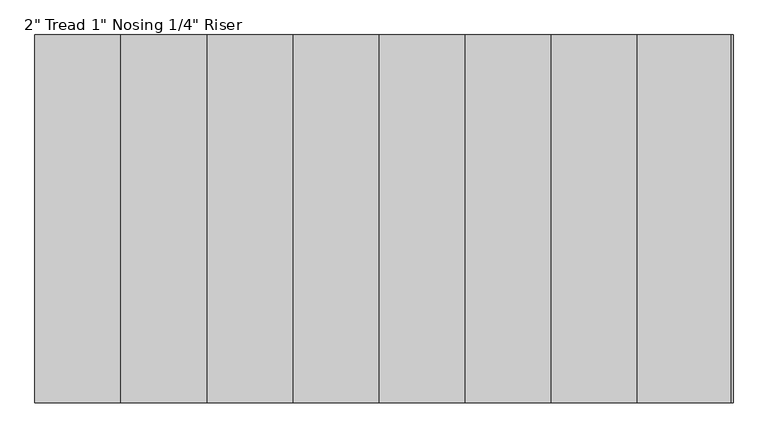
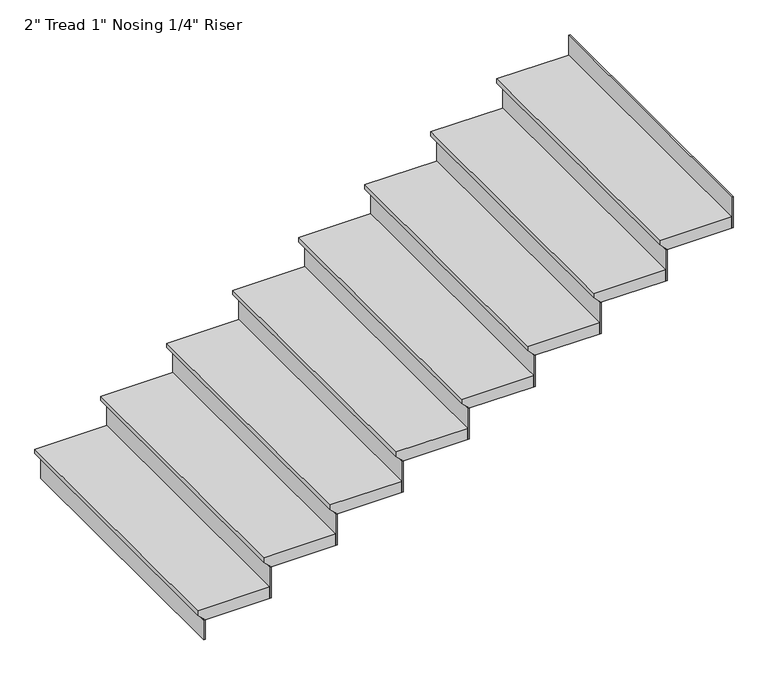
"""IFC4 building model written with IfcOpenShell, lengths in millimetres: stair flight geometry."""

from ifc_helpers import new_model, si_unit, origin, place, context, project, spatial, faceted_brep, source, transform, mapped, element, save


def stair_flight_e1fa31a4(model_context):
    return source(origin(), model_context, "Body", "Brep", [
        faceted_brep([(-12169.2183666, 2189.9503619, 3598.7934783), (-12169.2183666, 2189.9503619, 3617.8434783), (-12169.2183666, 3383.7503619, 3617.8434783), (-12169.2183666, 3383.7503619, 3598.7934783), (-12143.8183666, 2189.9503619, 3573.3934783), (-12143.8183666, 3383.7503619, 3573.3934783), (-11864.4183666, 2189.9503619, 3617.8434783), (-11864.4183666, 3383.7503619, 3617.8434783), (-12143.8183666, 3383.7503619, 3567.0434783), (-11864.4183666, 3383.7503619, 3567.0434783), (-11864.4183666, 2189.9503619, 3567.0434783), (-12143.8183666, 2189.9503619, 3567.0434783)], [[[0, 1, 2, 3]], [[4, 0, 3, 5]], [[2, 1, 6, 7]], [[8, 9, 10, 11]], [[2, 7, 9, 8, 5, 3]], [[8, 11, 4, 5]], [[6, 1, 0, 4, 11, 10]], [[7, 6, 10, 9]]]),
        faceted_brep([(-12143.8183666, 2189.9503619, 3567.0434783), (-12143.8183666, 2189.9503619, 3478.6956522), (-12137.4683666, 2189.9503619, 3478.6956522), (-12137.4683666, 2189.9503619, 3567.0434783), (-12143.8183666, 3383.7503619, 3567.0434783), (-12137.4683666, 3383.7503619, 3567.0434783), (-12137.4683666, 3383.7503619, 3478.6956522), (-12143.8183666, 3383.7503619, 3478.6956522)], [[[0, 1, 2, 3]], [[4, 5, 6, 7]], [[1, 0, 4, 7]], [[2, 1, 7, 6]], [[3, 2, 6, 5]], [[0, 3, 5, 4]]]),
        faceted_brep([(-11864.4183666, 2189.9503619, 3706.1913043), (-11864.4183666, 2189.9503619, 3567.0434783), (-11858.0683666, 2189.9503619, 3567.0434783), (-11858.0683666, 2189.9503619, 3706.1913043), (-11864.4183666, 3383.7503619, 3706.1913043), (-11858.0683666, 3383.7503619, 3706.1913043), (-11858.0683666, 3383.7503619, 3567.0434783), (-11864.4183666, 3383.7503619, 3567.0434783)], [[[0, 1, 2, 3]], [[4, 5, 6, 7]], [[1, 0, 4, 7]], [[2, 1, 7, 6]], [[3, 2, 6, 5]], [[0, 3, 5, 4]]]),
        faceted_brep([(-11889.8183666, 3383.7503619, 3756.9913043), (-11889.8183666, 2189.9503619, 3756.9913043), (-11585.0183666, 2189.9503619, 3756.9913043), (-11585.0183666, 3383.7503619, 3756.9913043), (-11864.4183666, 3383.7503619, 3706.1913043), (-11585.0183666, 3383.7503619, 3706.1913043), (-11585.0183666, 2189.9503619, 3706.1913043), (-11864.4183666, 2189.9503619, 3706.1913043), (-11864.4183666, 3383.7503619, 3712.5413043), (-11889.8183666, 3383.7503619, 3737.9413043), (-11864.4183666, 2189.9503619, 3712.5413043), (-11889.8183666, 2189.9503619, 3737.9413043)], [[[0, 1, 2, 3]], [[4, 5, 6, 7]], [[0, 3, 5, 4, 8, 9]], [[4, 7, 10, 8]], [[2, 1, 11, 10, 7, 6]], [[3, 2, 6, 5]], [[11, 1, 0, 9]], [[10, 11, 9, 8]]]),
        faceted_brep([(-11585.0183666, 2189.9503619, 3845.3391304), (-11585.0183666, 2189.9503619, 3706.1913043), (-11578.6683666, 2189.9503619, 3706.1913043), (-11578.6683666, 2189.9503619, 3845.3391304), (-11585.0183666, 3383.7503619, 3845.3391304), (-11578.6683666, 3383.7503619, 3845.3391304), (-11578.6683666, 3383.7503619, 3706.1913043), (-11585.0183666, 3383.7503619, 3706.1913043)], [[[0, 1, 2, 3]], [[4, 5, 6, 7]], [[1, 0, 4, 7]], [[2, 1, 7, 6]], [[3, 2, 6, 5]], [[0, 3, 5, 4]]]),
        faceted_brep([(-11610.4183666, 3383.7503619, 3896.1391304), (-11610.4183666, 2189.9503619, 3896.1391304), (-11305.6183666, 2189.9503619, 3896.1391304), (-11305.6183666, 3383.7503619, 3896.1391304), (-11585.0183666, 3383.7503619, 3845.3391304), (-11305.6183666, 3383.7503619, 3845.3391304), (-11305.6183666, 2189.9503619, 3845.3391304), (-11585.0183666, 2189.9503619, 3845.3391304), (-11585.0183666, 3383.7503619, 3851.6891304), (-11610.4183666, 3383.7503619, 3877.0891304), (-11585.0183666, 2189.9503619, 3851.6891304), (-11610.4183666, 2189.9503619, 3877.0891304)], [[[0, 1, 2, 3]], [[4, 5, 6, 7]], [[0, 3, 5, 4, 8, 9]], [[4, 7, 10, 8]], [[2, 1, 11, 10, 7, 6]], [[3, 2, 6, 5]], [[11, 1, 0, 9]], [[10, 11, 9, 8]]]),
        faceted_brep([(-11305.6183666, 2189.9503619, 3984.4869565), (-11305.6183666, 2189.9503619, 3845.3391304), (-11299.2683666, 2189.9503619, 3845.3391304), (-11299.2683666, 2189.9503619, 3984.4869565), (-11305.6183666, 3383.7503619, 3984.4869565), (-11299.2683666, 3383.7503619, 3984.4869565), (-11299.2683666, 3383.7503619, 3845.3391304), (-11305.6183666, 3383.7503619, 3845.3391304)], [[[0, 1, 2, 3]], [[4, 5, 6, 7]], [[1, 0, 4, 7]], [[2, 1, 7, 6]], [[3, 2, 6, 5]], [[0, 3, 5, 4]]]),
        faceted_brep([(-11331.0183666, 3383.7503619, 4035.2869565), (-11331.0183666, 2189.9503619, 4035.2869565), (-11026.2183666, 2189.9503619, 4035.2869565), (-11026.2183666, 3383.7503619, 4035.2869565), (-11305.6183666, 3383.7503619, 3984.4869565), (-11026.2183666, 3383.7503619, 3984.4869565), (-11026.2183666, 2189.9503619, 3984.4869565), (-11305.6183666, 2189.9503619, 3984.4869565), (-11305.6183666, 3383.7503619, 3990.8369565), (-11331.0183666, 3383.7503619, 4016.2369565), (-11305.6183666, 2189.9503619, 3990.8369565), (-11331.0183666, 2189.9503619, 4016.2369565)], [[[0, 1, 2, 3]], [[4, 5, 6, 7]], [[0, 3, 5, 4, 8, 9]], [[4, 7, 10, 8]], [[2, 1, 11, 10, 7, 6]], [[3, 2, 6, 5]], [[11, 1, 0, 9]], [[10, 11, 9, 8]]]),
        faceted_brep([(-11026.2183666, 2189.9503619, 4123.6347826), (-11026.2183666, 2189.9503619, 3984.4869565), (-11019.8683666, 2189.9503619, 3984.4869565), (-11019.8683666, 2189.9503619, 4123.6347826), (-11026.2183666, 3383.7503619, 4123.6347826), (-11019.8683666, 3383.7503619, 4123.6347826), (-11019.8683666, 3383.7503619, 3984.4869565), (-11026.2183666, 3383.7503619, 3984.4869565)], [[[0, 1, 2, 3]], [[4, 5, 6, 7]], [[1, 0, 4, 7]], [[2, 1, 7, 6]], [[3, 2, 6, 5]], [[0, 3, 5, 4]]]),
        faceted_brep([(-11051.6183666, 3383.7503619, 4174.4347826), (-11051.6183666, 2189.9503619, 4174.4347826), (-10746.8183666, 2189.9503619, 4174.4347826), (-10746.8183666, 3383.7503619, 4174.4347826), (-11026.2183666, 3383.7503619, 4123.6347826), (-10746.8183666, 3383.7503619, 4123.6347826), (-10746.8183666, 2189.9503619, 4123.6347826), (-11026.2183666, 2189.9503619, 4123.6347826), (-11026.2183666, 3383.7503619, 4129.9847826), (-11051.6183666, 3383.7503619, 4155.3847826), (-11026.2183666, 2189.9503619, 4129.9847826), (-11051.6183666, 2189.9503619, 4155.3847826)], [[[0, 1, 2, 3]], [[4, 5, 6, 7]], [[0, 3, 5, 4, 8, 9]], [[4, 7, 10, 8]], [[2, 1, 11, 10, 7, 6]], [[3, 2, 6, 5]], [[11, 1, 0, 9]], [[10, 11, 9, 8]]]),
        faceted_brep([(-10746.8183666, 2189.9503619, 4262.7826087), (-10746.8183666, 2189.9503619, 4123.6347826), (-10740.4683666, 2189.9503619, 4123.6347826), (-10740.4683666, 2189.9503619, 4262.7826087), (-10746.8183666, 3383.7503619, 4262.7826087), (-10740.4683666, 3383.7503619, 4262.7826087), (-10740.4683666, 3383.7503619, 4123.6347826), (-10746.8183666, 3383.7503619, 4123.6347826)], [[[0, 1, 2, 3]], [[4, 5, 6, 7]], [[1, 0, 4, 7]], [[2, 1, 7, 6]], [[3, 2, 6, 5]], [[0, 3, 5, 4]]]),
        faceted_brep([(-10772.2183666, 3383.7503619, 4313.5826087), (-10772.2183666, 2189.9503619, 4313.5826087), (-10467.4183666, 2189.9503619, 4313.5826087), (-10467.4183666, 3383.7503619, 4313.5826087), (-10746.8183666, 3383.7503619, 4262.7826087), (-10467.4183666, 3383.7503619, 4262.7826087), (-10467.4183666, 2189.9503619, 4262.7826087), (-10746.8183666, 2189.9503619, 4262.7826087), (-10746.8183666, 3383.7503619, 4269.1326087), (-10772.2183666, 3383.7503619, 4294.5326087), (-10746.8183666, 2189.9503619, 4269.1326087), (-10772.2183666, 2189.9503619, 4294.5326087)], [[[0, 1, 2, 3]], [[4, 5, 6, 7]], [[0, 3, 5, 4, 8, 9]], [[4, 7, 10, 8]], [[2, 1, 11, 10, 7, 6]], [[3, 2, 6, 5]], [[11, 1, 0, 9]], [[10, 11, 9, 8]]]),
        faceted_brep([(-10467.4183666, 2189.9503619, 4401.9304348), (-10467.4183666, 2189.9503619, 4262.7826087), (-10461.0683666, 2189.9503619, 4262.7826087), (-10461.0683666, 2189.9503619, 4401.9304348), (-10467.4183666, 3383.7503619, 4401.9304348), (-10461.0683666, 3383.7503619, 4401.9304348), (-10461.0683666, 3383.7503619, 4262.7826087), (-10467.4183666, 3383.7503619, 4262.7826087)], [[[0, 1, 2, 3]], [[4, 5, 6, 7]], [[1, 0, 4, 7]], [[2, 1, 7, 6]], [[3, 2, 6, 5]], [[0, 3, 5, 4]]]),
        faceted_brep([(-10492.8183666, 3383.7503619, 4452.7304348), (-10492.8183666, 2189.9503619, 4452.7304348), (-10188.0183666, 2189.9503619, 4452.7304348), (-10188.0183666, 3383.7503619, 4452.7304348), (-10467.4183666, 3383.7503619, 4401.9304348), (-10188.0183666, 3383.7503619, 4401.9304348), (-10188.0183666, 2189.9503619, 4401.9304348), (-10467.4183666, 2189.9503619, 4401.9304348), (-10467.4183666, 3383.7503619, 4408.2804348), (-10492.8183666, 3383.7503619, 4433.6804348), (-10467.4183666, 2189.9503619, 4408.2804348), (-10492.8183666, 2189.9503619, 4433.6804348)], [[[0, 1, 2, 3]], [[4, 5, 6, 7]], [[0, 3, 5, 4, 8, 9]], [[4, 7, 10, 8]], [[2, 1, 11, 10, 7, 6]], [[3, 2, 6, 5]], [[11, 1, 0, 9]], [[10, 11, 9, 8]]]),
        faceted_brep([(-10188.0183666, 2189.9503619, 4541.0782609), (-10188.0183666, 2189.9503619, 4401.9304348), (-10181.6683666, 2189.9503619, 4401.9304348), (-10181.6683666, 2189.9503619, 4541.0782609), (-10188.0183666, 3383.7503619, 4541.0782609), (-10181.6683666, 3383.7503619, 4541.0782609), (-10181.6683666, 3383.7503619, 4401.9304348), (-10188.0183666, 3383.7503619, 4401.9304348)], [[[0, 1, 2, 3]], [[4, 5, 6, 7]], [[1, 0, 4, 7]], [[2, 1, 7, 6]], [[3, 2, 6, 5]], [[0, 3, 5, 4]]]),
        faceted_brep([(-9908.6183666, 2189.9503619, 4680.226087), (-9908.6183666, 2189.9503619, 4541.0782609), (-9902.2683666, 2189.9503619, 4541.0782609), (-9902.2683666, 2189.9503619, 4680.226087), (-9908.6183666, 3383.7503619, 4680.226087), (-9902.2683666, 3383.7503619, 4680.226087), (-9902.2683666, 3383.7503619, 4541.0782609), (-9908.6183666, 3383.7503619, 4541.0782609)], [[[0, 1, 2, 3]], [[4, 5, 6, 7]], [[1, 0, 4, 7]], [[2, 1, 7, 6]], [[3, 2, 6, 5]], [[0, 3, 5, 4]]]),
        faceted_brep([(-9908.6183666, 3383.7503619, 4591.8782609), (-9934.0183666, 3383.7503619, 4591.8782609), (-10213.4183666, 3383.7503619, 4591.8782609), (-10213.4183666, 2189.9503619, 4591.8782609), (-9908.6183666, 2189.9503619, 4591.8782609), (-9934.0183666, 3383.7503619, 4541.0782609), (-9908.6183666, 3383.7503619, 4541.0782609), (-9908.6183666, 2189.9503619, 4541.0782609), (-10188.0183666, 2189.9503619, 4541.0782609), (-10188.0183666, 3383.7503619, 4541.0782609), (-10188.0183666, 3383.7503619, 4547.4282609), (-10213.4183666, 3383.7503619, 4572.8282609), (-10188.0183666, 2189.9503619, 4547.4282609), (-10213.4183666, 2189.9503619, 4572.8282609)], [[[0, 1, 2, 3, 4]], [[5, 6, 7, 8, 9]], [[1, 0, 6, 5]], [[2, 1, 5, 9, 10, 11]], [[9, 8, 12, 10]], [[4, 3, 13, 12, 8, 7]], [[0, 4, 7, 6]], [[13, 3, 2, 11]], [[12, 13, 11, 10]]]),
    ])


if __name__ == "__main__":
    model = new_model("IFC4")
    model_context = context("Model", 3, world=origin())
    ifc_project = project(units=[si_unit("LENGTHUNIT", "METRE", prefix="MILLI")], contexts=[model_context])
    site = spatial("IfcSite", under=ifc_project)
    building = spatial("IfcBuilding", under=site)
    placement = place(None, origin())
    stair_flight_shape = stair_flight_e1fa31a4(model_context)
    element("IfcStairFlight", 1, ObjectType="2\" Tread 1\" Nosing 1/4\" Riser", at=placement, inside=building, context=model_context, shape_type="MappedRepresentation", body=[
        mapped(stair_flight_shape, transform((0.0, 0.0, 0.0), x_axis=(1.0, 0.0, 0.0), y_axis=(0.0, 1.0, 0.0), z_axis=(0.0, 0.0, 1.0))),
    ])
    save(model, "model.ifc")
